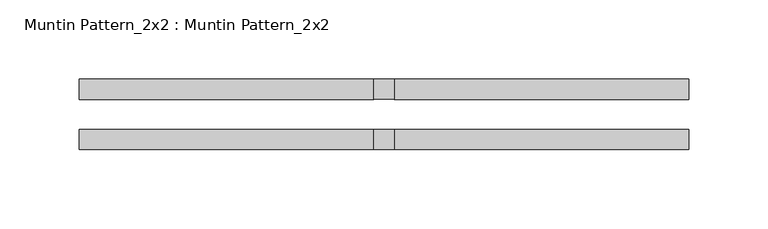
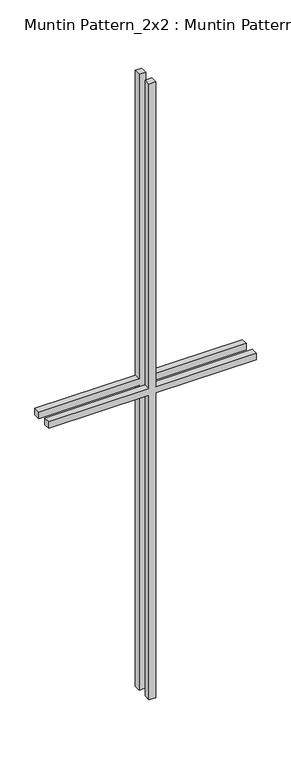
"""IFC4 building model written with IfcOpenShell, lengths in millimetres: proxy geometry, Muntin Pattern_2x2 : Muntin Pattern_2x2."""

from ifc_helpers import new_model, si_unit, frame, origin, place, context, project, spatial, polyline, outline, extrude, source, transform, mapped, element, save


def muntin_pattern_2x2_muntin_pattern_2x2_88bf7f41(model_context):
    return source(origin(), model_context, "Body", "SweptSolid", [
        extrude(outline(polyline([(609.6, -6.35), (609.6, -192.0875), (596.9, -192.0875), (596.9, -6.35), (0.0, -6.35), (0.0, 6.35), (596.9, 6.35), (596.9, 192.0875), (609.6, 192.0875), (609.6, 6.35), (1206.5, 6.35), (1206.5, -6.35), (609.6, -6.35)])), frame((0.0, 9.525, 0.0), z_axis=(0.0, 1.0, 0.0), x_axis=(0.0, 0.0, 1.0)), (0.0, 0.0, 1.0), 12.7),
        extrude(outline(polyline([(609.6, -6.35), (609.6, -192.0875), (596.9, -192.0875), (596.9, -6.35), (0.0, -6.35), (0.0, 6.35), (596.9, 6.35), (596.9, 192.0875), (609.6, 192.0875), (609.6, 6.35), (1206.5, 6.35), (1206.5, -6.35), (609.6, -6.35)])), frame((0.0, -22.225, 0.0), z_axis=(0.0, 1.0, 0.0), x_axis=(0.0, 0.0, 1.0)), (0.0, 0.0, 1.0), 12.7),
    ])


if __name__ == "__main__":
    model = new_model("IFC4")
    model_context = context("Model", 3, world=origin())
    ifc_project = project(units=[si_unit("LENGTHUNIT", "METRE", prefix="MILLI")], contexts=[model_context])
    site = spatial("IfcSite", under=ifc_project)
    building = spatial("IfcBuilding", under=site)
    placement = place(None, origin())
    muntin_pattern_2x2_muntin_pattern_2x2_shape = muntin_pattern_2x2_muntin_pattern_2x2_88bf7f41(model_context)
    element("IfcBuildingElementProxy", 1, Name="Muntin Pattern_2x2 : Muntin Pattern_2x2", ObjectType="Muntin Pattern_2x2 : Muntin Pattern_2x2", at=placement, inside=building, context=model_context, shape_type="MappedRepresentation", body=[
        mapped(muntin_pattern_2x2_muntin_pattern_2x2_shape, transform((0.0, 0.0, 0.0), x_axis=(1.0, 0.0, 0.0), y_axis=(0.0, 1.0, 0.0), z_axis=(0.0, 0.0, 1.0))),
    ])
    save(model, "model.ifc")

# Revit data of these elements
# Type "Muntin Pattern_2x2 : Muntin Pattern_2x2"
#   Width [instance default] = 4' - 0"
#   Thickness = 0' - 0 1/2"
#   Height [instance default] = 4' - 0"
#   Distance = 0' - 0 3/4"
#   Interior Material [instance default] = none
#   Exterior Material [instance default] = none
#   Default Elevation = 0
# Element 1 (IfcBuildingElementProxy, "Muntin Pattern_2x2 : Muntin Pattern_2x2")
#   Width = 1' - 3 1/8"
#   Height = 3' - 11 1/2"
#   Interior Material = Wood - Stained
#   Exterior Material = Clad - White
#   Materials on its faces: "Clad - White", "Wood - Stained"
# Materials
#   "Clad - White": class "Wood", colour RGB 242 242 238, transparency 0, Cost = 0
#   "Wood - Stained": class "Wood", colour RGB 224 178 126, transparency 0, Cost = 0
